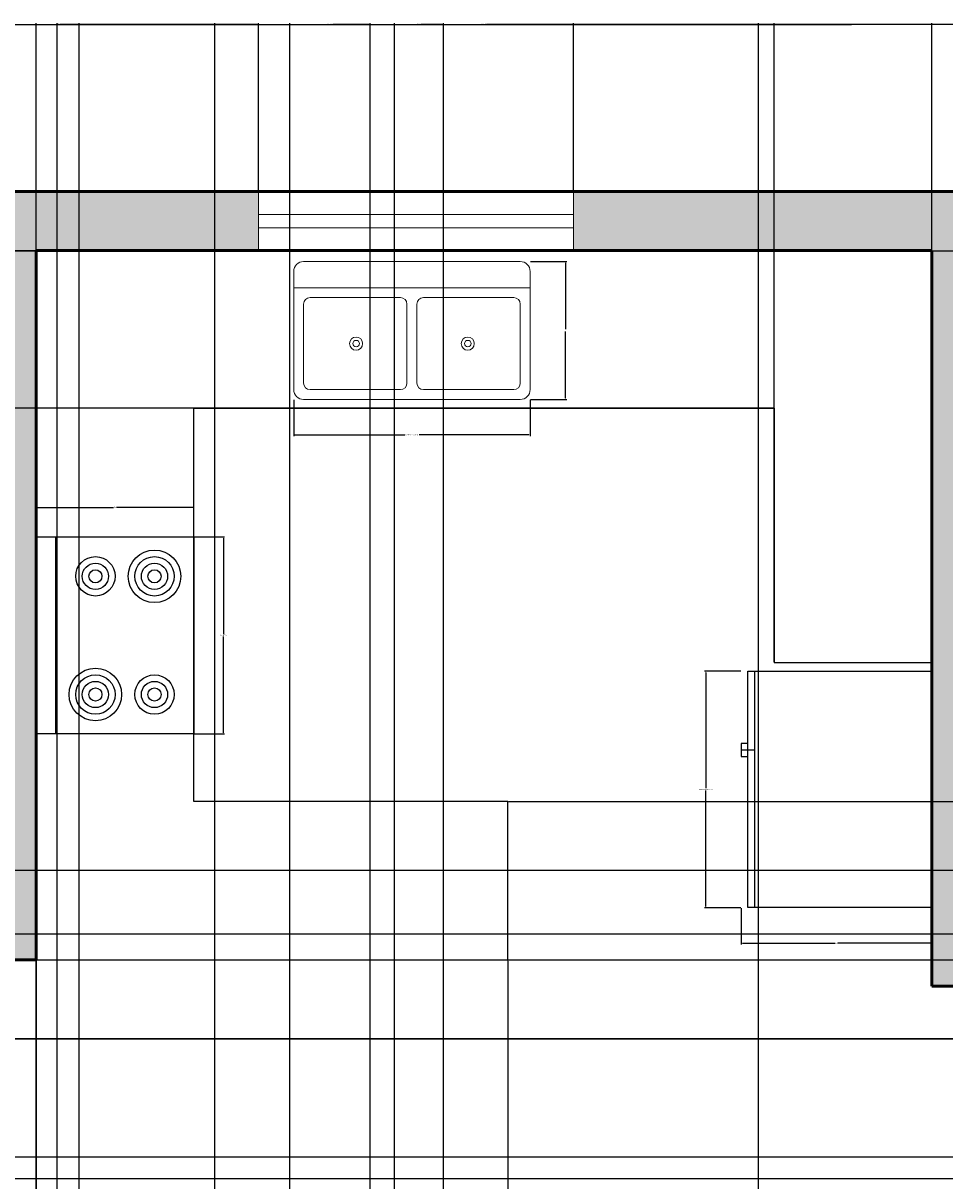
# Model space of a CAD drawing. Units: inches. Extents: x 3439 to 3988, y 1915 to 2284.
# Tile 6 of 7: x 3656 to 3796, y 2108 to 2284. Entities that reach past the tile are written whole.
import ezdxf

# ---------------------------------------------------------------- set-up
doc = ezdxf.new("R2010")
doc.units = ezdxf.units.IN
for name, color, linetype, lineweight in [('A-ANNO-DIMS', 2, 'Continuous', 18), ('A-EQPM', 8, 'Continuous', 25), ('A-FLOR-CASE', 8, 'Continuous', 25), ('A-FLOR-FIXT', 9, 'Continuous', 18), ('A-GLAZ', 4, 'Continuous', 18), ('A-WALL', 7, 'Continuous', 50)]:
    doc.layers.add(name, color=color, linetype=linetype, lineweight=lineweight)
doc.layers.add('A-WALL-PATT', color=18, linetype='Continuous', lineweight=13, true_color=0x000000)
doc.styles.get("Standard").update_dxf_attribs({"font": 'arial.ttf'})
doc.dimstyles.get("Standard").update_dxf_attribs({"dimtxt": 0.18, "dimasz": 0.18, "dimexe": 0.18, "dimexo": 0.0625, "dimgap": 0.09, "dimtad": 0, "dimtih": 1, "dimtoh": 1, "dimdec": 4, "dimzin": 0, "dimdsep": 46, "dimtxsty": 'Standard', "dimcen": 0.09, "dimadec": 0, "dimazin": 0, "dimtfac": 1, "dimtdec": 4, "dimtofl": 0, "dimtmove": 0, "dimatfit": 3, "dimfxl": 1, "dimtolj": 1, "dimtzin": 0, "dimarcsym": 0})

# ---------------------------------------------------------------- blocks, each defined once
blk = doc.blocks.new('Range-Oven - 30 in top')
blk.add_line((0, -3), (30, -3))
blk.add_lwpolyline([(0, -24), (0, 0), (30, 0), (30, -24)], close=True)
for centre, radius in [((6, -9), 4), ((6, -9), 3), ((6, -9), 2), ((24, -9), 3), ((24, -9), 2), ((6, -9), 1), ((24, -9), 1), ((24, -18), 4), ((6, -18), 3), ((24, -18), 3), ((6, -18), 2), ((6, -18), 1), ((24, -18), 2), ((24, -18), 1)]:
    blk.add_circle(centre, radius)
blk = doc.blocks.new('Sink-double - 36 in top')
for p, q in [((-18, -4), (18, -4)), ((-0.75, -18.5), (-0.75, -6.5)), ((0.75, -6.5), (0.75, -18.5))]:
    blk.add_line(p, q)
for points in [[(-16.5, 0), (16.5, 0)], [(-18, -19.5), (-18, -1.5)], [(18, -1.5), (18, -19.5)], [(-16.5, -18.5), (-16.5, -6.5)], [(-15.5, -5.5), (-1.75, -5.5)], [(1.75, -5.5), (15.5, -5.5)], [(16.5, -6.5), (16.5, -18.5)], [(16.5, -21), (-16.5, -21)], [(-1.75, -19.5), (-15.5, -19.5)], [(15.5, -19.5), (1.75, -19.5)]]:
    blk.add_lwpolyline(points)
for centre, radius in [((-8.5, -12.5), 1), ((-8.5, -12.5), 0.5), ((8.5, -12.5), 1), ((8.5, -12.5), 0.5)]:
    blk.add_circle(centre, radius)
for centre, radius, start, end in [((-16.5, -1.5), 1.5, 90, 180), ((16.5, -1.5), 1.5, 0, 90), ((-15.5, -6.5), 1, 90, 180), ((-1.75, -6.5), 1, 0, 90), ((1.75, -6.5), 1, 90, 180), ((15.5, -6.5), 1, 0, 90), ((-15.5, -18.5), 1, 180, 270), ((-1.75, -18.5), 1, 270, 0), ((1.75, -18.5), 1, 180, 270), ((15.5, -18.5), 1, 270, 0), ((-16.5, -19.5), 1.5, 180, 270), ((16.5, -19.5), 1.5, 270, 0)]:
    blk.add_arc(centre, radius, start, end)
blk = doc.blocks.new('Refrigerator-2 door - 36 in top')
for p, q in [((0, -26.999999), (36, -26.999999)), ((11, -27.999999), (11, -28.999999)), ((12, -26.999999), (12, -28.999999)), ((13, -28.999999), (13, -27.999999)), ((11, -28.999999), (13, -28.999999))]:
    blk.add_line(p, q)
blk.add_lwpolyline([(0, -27.999999), (0, 0), (36, 0), (36, -27.999999)], close=True)
blk = doc.blocks.new('WINDOW-GLASS-48IN')
for p, q in [((0, 2), (48, 2)), ((0, 0), (48, 0))]:
    blk.add_line(p, q)
blk = doc.blocks.new('*D37')
at = {"layer": 'A-ANNO-DIMS', "color": 0, "lineweight": -2, "transparency": 16777216}
for p, q in [((3681.64, 2205.78), (3686.26, 2205.78)), ((3686.08, 2205.6), (3686.08, 2190.96)), ((3686.08, 2175.96), (3686.08, 2190.59)), ((3681.64, 2175.78), (3686.26, 2175.78))]:
    blk.add_line(p, q, dxfattribs=at)
at = {"layer": 'A-ANNO-DIMS', "color": 0, "transparency": 16777216}
for points in [[(3686.05, 2205.6), (3686.11, 2205.6), (3686.08, 2205.78)], [(3686.05, 2175.96), (3686.11, 2175.96), (3686.08, 2175.78)]]:
    blk.add_solid(points, dxfattribs=at)
at = {"layer": 'Defpoints', "color": 0, "transparency": 16777216}
for p in [(3681.58, 2205.78), (3686.08, 2205.78), (3681.58, 2175.78)]:
    blk.add_point(p, dxfattribs=at)
at = {"layer": 'A-ANNO-DIMS', "color": 0, "transparency": 16777216, "insert": (3686.08, 2190.78), "char_height": 0.18, "attachment_point": 5}
blk.add_mtext('\\A1;RANGE 30', dxfattribs=at)
blk = doc.blocks.new('*D38')
at = {"layer": 'A-ANNO-DIMS', "color": 0, "lineweight": -2, "transparency": 16777216}
for p, q in [((3657.58, 2205.84), (3657.58, 2210.46)), ((3657.76, 2210.28), (3669.36, 2210.28)), ((3681.4, 2210.28), (3669.8, 2210.28)), ((3681.58, 2205.84), (3681.58, 2210.46))]:
    blk.add_line(p, q, dxfattribs=at)
at = {"layer": 'A-ANNO-DIMS', "color": 0, "transparency": 16777216}
for points in [[(3657.76, 2210.31), (3657.76, 2210.25), (3657.58, 2210.28)], [(3681.4, 2210.31), (3681.4, 2210.25), (3681.58, 2210.28)]]:
    blk.add_solid(points, dxfattribs=at)
at = {"layer": 'Defpoints', "color": 0, "transparency": 16777216}
for p in [(3657.58, 2210.28), (3657.58, 2205.78), (3681.58, 2205.78)]:
    blk.add_point(p, dxfattribs=at)
at = {"layer": 'A-ANNO-DIMS', "color": 0, "transparency": 16777216, "insert": (3669.58, 2210.28), "char_height": 0.18, "attachment_point": 5}
blk.add_mtext('\\A1;24', dxfattribs=at)
blk = doc.blocks.new('*D39')
at = {"layer": 'A-ANNO-DIMS', "color": 0, "lineweight": -2, "transparency": 16777216}
for p, q in [((3696.78, 2226.64), (3696.78, 2221.13)), ((3732.78, 2226.64), (3732.78, 2221.13)), ((3696.96, 2221.31), (3713.69, 2221.31)), ((3732.6, 2221.31), (3715.87, 2221.31))]:
    blk.add_line(p, q, dxfattribs=at)
at = {"layer": 'A-ANNO-DIMS', "color": 0, "transparency": 16777216}
for points in [[(3696.96, 2221.34), (3696.96, 2221.28), (3696.78, 2221.31)], [(3732.6, 2221.34), (3732.6, 2221.28), (3732.78, 2221.31)]]:
    blk.add_solid(points, dxfattribs=at)
at = {"layer": 'Defpoints', "color": 0, "transparency": 16777216}
for p in [(3696.78, 2226.71), (3732.78, 2226.71), (3732.78, 2221.31)]:
    blk.add_point(p, dxfattribs=at)
at = {"layer": 'A-ANNO-DIMS', "color": 0, "transparency": 16777216, "insert": (3714.78, 2221.31), "char_height": 0.18, "attachment_point": 5}
blk.add_mtext('\\A1;DOUBLE SINK 36', dxfattribs=at)
blk = doc.blocks.new('*D40')
at = {"layer": 'A-ANNO-DIMS', "color": 0, "lineweight": -2, "transparency": 16777216}
for p, q in [((3732.84, 2247.71), (3738.36, 2247.71)), ((3738.18, 2247.53), (3738.18, 2237.39)), ((3738.18, 2226.89), (3738.18, 2237.03)), ((3732.84, 2226.71), (3738.36, 2226.71))]:
    blk.add_line(p, q, dxfattribs=at)
at = {"layer": 'A-ANNO-DIMS', "color": 0, "transparency": 16777216}
for points in [[(3738.15, 2247.53), (3738.21, 2247.53), (3738.18, 2247.71)], [(3738.15, 2226.89), (3738.21, 2226.89), (3738.18, 2226.71)]]:
    blk.add_solid(points, dxfattribs=at)
at = {"layer": 'Defpoints', "color": 0, "transparency": 16777216}
for p in [(3732.78, 2247.71), (3738.18, 2247.71), (3732.78, 2226.71)]:
    blk.add_point(p, dxfattribs=at)
at = {"layer": 'A-ANNO-DIMS', "color": 0, "transparency": 16777216, "insert": (3738.18, 2237.21), "char_height": 0.18, "attachment_point": 5}
blk.add_mtext('\\A1;21', dxfattribs=at)
blk = doc.blocks.new('*D43')
at = {"layer": 'A-ANNO-DIMS', "color": 0, "lineweight": -2, "transparency": 16777216}
for p, q in [((3764.87, 2185.32), (3759.35, 2185.32)), ((3759.53, 2185.14), (3759.53, 2167.51)), ((3759.53, 2149.5), (3759.53, 2167.14)), ((3764.87, 2149.32), (3759.35, 2149.32))]:
    blk.add_line(p, q, dxfattribs=at)
at = {"layer": 'A-ANNO-DIMS', "color": 0, "transparency": 16777216}
for points in [[(3759.5, 2185.14), (3759.56, 2185.14), (3759.53, 2185.32)], [(3759.5, 2149.5), (3759.56, 2149.5), (3759.53, 2149.32)]]:
    blk.add_solid(points, dxfattribs=at)
at = {"layer": 'Defpoints', "color": 0, "transparency": 16777216}
for p in [(3764.93, 2185.32), (3759.53, 2149.32), (3764.93, 2149.32)]:
    blk.add_point(p, dxfattribs=at)
at = {"layer": 'A-ANNO-DIMS', "color": 0, "transparency": 16777216, "insert": (3759.53, 2167.32), "char_height": 0.18, "attachment_point": 5}
blk.add_mtext('\\A1;REFRIGERATOR 36', dxfattribs=at)
blk = doc.blocks.new('*D44')
at = {"layer": 'A-ANNO-DIMS', "color": 0, "lineweight": -2, "transparency": 16777216}
for p, q in [((3764.93, 2149.26), (3764.93, 2143.74)), ((3793.93, 2149.26), (3793.93, 2143.74)), ((3765.11, 2143.92), (3779.21, 2143.92)), ((3793.75, 2143.92), (3779.65, 2143.92))]:
    blk.add_line(p, q, dxfattribs=at)
at = {"layer": 'A-ANNO-DIMS', "color": 0, "transparency": 16777216}
for points in [[(3765.11, 2143.95), (3765.11, 2143.89), (3764.93, 2143.92)], [(3793.75, 2143.95), (3793.75, 2143.89), (3793.93, 2143.92)]]:
    blk.add_solid(points, dxfattribs=at)
at = {"layer": 'Defpoints', "color": 0, "transparency": 16777216}
for p in [(3764.93, 2149.32), (3793.93, 2149.32), (3793.93, 2143.92)]:
    blk.add_point(p, dxfattribs=at)
at = {"layer": 'A-ANNO-DIMS', "color": 0, "transparency": 16777216, "insert": (3779.43, 2143.92), "char_height": 0.18, "attachment_point": 5}
blk.add_mtext('\\A1;29', dxfattribs=at)
blk = doc.blocks.new('*D49')
at = {"layer": 'A-ANNO-DIMS', "color": 0, "lineweight": -2, "transparency": 16777216}
for p, q in [((3657.58, 2249.42), (3657.58, 2284)), ((3657.76, 2283.82), (3725.3, 2283.82)), ((3793.75, 2283.82), (3726.21, 2283.82)), ((3793.93, 2249.42), (3793.93, 2284))]:
    blk.add_line(p, q, dxfattribs=at)
at = {"layer": 'A-ANNO-DIMS', "color": 0, "transparency": 16777216}
for points in [[(3657.76, 2283.85), (3657.76, 2283.79), (3657.58, 2283.82)], [(3793.75, 2283.85), (3793.75, 2283.79), (3793.93, 2283.82)]]:
    blk.add_solid(points, dxfattribs=at)
at = {"layer": 'Defpoints', "color": 0, "transparency": 16777216}
for p in [(3793.93, 2283.82), (3657.58, 2249.36), (3793.93, 2249.36)]:
    blk.add_point(p, dxfattribs=at)
at = {"layer": 'A-ANNO-DIMS', "color": 0, "transparency": 16777216, "insert": (3725.76, 2283.82), "char_height": 0.18, "attachment_point": 5}
blk.add_mtext('\\A1;136.35', dxfattribs=at)
blk = doc.blocks.new('*D64')
at = {"layer": 'A-ANNO-DIMS', "color": 0, "lineweight": -2, "transparency": 16777216}
for p, q in [((3593.64, 2249.36), (3987.81, 2249.36)), ((3987.63, 2249.18), (3987.63, 2197.54)), ((3987.63, 2145.54), (3987.63, 2197.18)), ((3593.64, 2145.36), (3987.81, 2145.36))]:
    blk.add_line(p, q, dxfattribs=at)
at = {"layer": 'A-ANNO-DIMS', "color": 0, "transparency": 16777216}
for points in [[(3987.6, 2249.18), (3987.66, 2249.18), (3987.63, 2249.36)], [(3987.6, 2145.54), (3987.66, 2145.54), (3987.63, 2145.36)]]:
    blk.add_solid(points, dxfattribs=at)
at = {"layer": 'Defpoints', "color": 0, "transparency": 16777216}
for p in [(3593.58, 2249.36), (3987.63, 2249.36), (3593.58, 2145.36)]:
    blk.add_point(p, dxfattribs=at)
at = {"layer": 'A-ANNO-DIMS', "color": 0, "transparency": 16777216, "insert": (3987.63, 2197.36), "char_height": 0.18, "attachment_point": 5}
blk.add_mtext('\\A1;104', dxfattribs=at)
blk = doc.blocks.new('*D68')
at = {"layer": 'A-ANNO-DIMS', "color": 0, "lineweight": -2, "transparency": 16777216}
for p, q in [((3631.59, 2258.42), (3631.59, 2284)), ((3631.77, 2283.82), (3661.12, 2283.82)), ((3691.23, 2283.82), (3661.88, 2283.82)), ((3691.41, 2258.42), (3691.41, 2284))]:
    blk.add_line(p, q, dxfattribs=at)
at = {"layer": 'A-ANNO-DIMS', "color": 0, "transparency": 16777216}
for points in [[(3631.77, 2283.85), (3631.77, 2283.79), (3631.59, 2283.82)], [(3691.23, 2283.85), (3691.23, 2283.79), (3691.41, 2283.82)]]:
    blk.add_solid(points, dxfattribs=at)
at = {"layer": 'Defpoints', "color": 0, "transparency": 16777216}
for p in [(3691.41, 2283.82), (3631.59, 2258.36), (3691.41, 2258.36)]:
    blk.add_point(p, dxfattribs=at)
at = {"layer": 'A-ANNO-DIMS', "color": 0, "transparency": 16777216, "insert": (3661.5, 2283.82), "char_height": 0.18, "attachment_point": 5}
blk.add_mtext('\\A1;59.81', dxfattribs=at)
blk = doc.blocks.new('*D69')
at = {"layer": 'A-ANNO-DIMS', "color": 0, "lineweight": -2, "transparency": 16777216}
for p, q in [((3739.41, 2258.42), (3739.41, 2284)), ((3739.59, 2283.82), (3771.27, 2283.82)), ((3803.75, 2283.82), (3772.06, 2283.82)), ((3803.93, 2258.42), (3803.93, 2284))]:
    blk.add_line(p, q, dxfattribs=at)
at = {"layer": 'A-ANNO-DIMS', "color": 0, "transparency": 16777216}
for points in [[(3739.59, 2283.85), (3739.59, 2283.79), (3739.41, 2283.82)], [(3803.75, 2283.85), (3803.75, 2283.79), (3803.93, 2283.82)]]:
    blk.add_solid(points, dxfattribs=at)
at = {"layer": 'Defpoints', "color": 0, "transparency": 16777216}
for p in [(3803.93, 2283.82), (3739.41, 2258.36), (3803.93, 2258.36)]:
    blk.add_point(p, dxfattribs=at)
at = {"layer": 'A-ANNO-DIMS', "color": 0, "transparency": 16777216, "insert": (3771.67, 2283.82), "char_height": 0.18, "attachment_point": 5}
blk.add_mtext('\\A1;64.53', dxfattribs=at)
blk = doc.blocks.new('*D73')
at = {"layer": 'A-ANNO-DIMS', "color": 0, "lineweight": -2, "transparency": 16777216}
for p, q in [((3657.58, 1949.42), (3657.58, 2284)), ((3657.76, 2283.82), (3660.52, 2283.82)), ((3663.93, 2283.82), (3661.17, 2283.82)), ((3664.11, 1949.42), (3664.11, 2284))]:
    blk.add_line(p, q, dxfattribs=at)
at = {"layer": 'A-ANNO-DIMS', "color": 0, "transparency": 16777216}
for points in [[(3657.76, 2283.85), (3657.76, 2283.79), (3657.58, 2283.82)], [(3663.93, 2283.85), (3663.93, 2283.79), (3664.11, 2283.82)]]:
    blk.add_solid(points, dxfattribs=at)
at = {"layer": 'Defpoints', "color": 0, "transparency": 16777216}
for p in [(3664.11, 2283.82), (3657.58, 1949.36), (3664.11, 1949.36)]:
    blk.add_point(p, dxfattribs=at)
at = {"layer": 'A-ANNO-DIMS', "color": 0, "transparency": 16777216, "insert": (3660.85, 2283.82), "char_height": 0.18, "attachment_point": 5}
blk.add_mtext('\\A1;6.53', dxfattribs=at)
blk = doc.blocks.new('*D74')
at = {"layer": 'A-ANNO-DIMS', "color": 0, "lineweight": -2, "transparency": 16777216}
for p, q in [((3712.11, 1949.42), (3712.11, 2284)), ((3712.29, 2283.82), (3715.52, 2283.82)), ((3719.4, 2283.82), (3716.17, 2283.82)), ((3719.58, 1949.42), (3719.58, 2284))]:
    blk.add_line(p, q, dxfattribs=at)
at = {"layer": 'A-ANNO-DIMS', "color": 0, "transparency": 16777216}
for points in [[(3712.29, 2283.85), (3712.29, 2283.79), (3712.11, 2283.82)], [(3719.4, 2283.85), (3719.4, 2283.79), (3719.58, 2283.82)]]:
    blk.add_solid(points, dxfattribs=at)
at = {"layer": 'Defpoints', "color": 0, "transparency": 16777216}
for p in [(3719.58, 2283.82), (3712.11, 1949.36), (3719.58, 1949.36)]:
    blk.add_point(p, dxfattribs=at)
at = {"layer": 'A-ANNO-DIMS', "color": 0, "transparency": 16777216, "insert": (3715.85, 2283.82), "char_height": 0.18, "attachment_point": 5}
blk.add_mtext('\\A1;7.47', dxfattribs=at)
blk = doc.blocks.new('*D75')
at = {"layer": 'A-ANNO-DIMS', "color": 0, "lineweight": -2, "transparency": 16777216}
for p, q in [((3719.58, 1949.42), (3719.58, 2284)), ((3719.76, 2283.82), (3743.36, 2283.82)), ((3767.4, 2283.82), (3743.8, 2283.82)), ((3767.58, 1949.42), (3767.58, 2284))]:
    blk.add_line(p, q, dxfattribs=at)
at = {"layer": 'A-ANNO-DIMS', "color": 0, "transparency": 16777216}
for points in [[(3719.76, 2283.85), (3719.76, 2283.79), (3719.58, 2283.82)], [(3767.4, 2283.85), (3767.4, 2283.79), (3767.58, 2283.82)]]:
    blk.add_solid(points, dxfattribs=at)
at = {"layer": 'Defpoints', "color": 0, "transparency": 16777216}
for p in [(3767.58, 2283.82), (3719.58, 1949.36), (3767.58, 1949.36)]:
    blk.add_point(p, dxfattribs=at)
at = {"layer": 'A-ANNO-DIMS', "color": 0, "transparency": 16777216, "insert": (3743.58, 2283.82), "char_height": 0.18, "attachment_point": 5}
blk.add_mtext('\\A1;48', dxfattribs=at)
blk = doc.blocks.new('*D77')
at = {"layer": 'A-ANNO-DIMS', "color": 0, "lineweight": -2, "transparency": 16777216}
for p, q in [((3473.64, 2129.36), (3987.81, 2129.36)), ((3987.63, 2129.18), (3987.63, 2118.9)), ((3987.63, 2108.25), (3987.63, 2118.53)), ((3473.64, 2108.07), (3987.81, 2108.07))]:
    blk.add_line(p, q, dxfattribs=at)
at = {"layer": 'A-ANNO-DIMS', "color": 0, "transparency": 16777216}
for points in [[(3987.6, 2129.18), (3987.66, 2129.18), (3987.63, 2129.36)], [(3987.6, 2108.25), (3987.66, 2108.25), (3987.63, 2108.07)]]:
    blk.add_solid(points, dxfattribs=at)
at = {"layer": 'Defpoints', "color": 0, "transparency": 16777216}
for p in [(3473.58, 2129.36), (3987.63, 2129.36), (3473.58, 2108.07)]:
    blk.add_point(p, dxfattribs=at)
at = {"layer": 'A-ANNO-DIMS', "color": 0, "transparency": 16777216, "insert": (3987.63, 2118.71), "char_height": 0.18, "attachment_point": 5}
blk.add_mtext('\\A1;21.295', dxfattribs=at)
blk = doc.blocks.new('*D82')
at = {"layer": 'A-ANNO-DIMS', "color": 0, "lineweight": -2, "transparency": 16777216}
for p, q in [((3537.64, 2129.36), (3987.81, 2129.36)), ((3987.63, 2129.18), (3987.63, 2120.54)), ((3987.63, 2111.54), (3987.63, 2120.18)), ((3537.64, 2111.36), (3987.81, 2111.36))]:
    blk.add_line(p, q, dxfattribs=at)
at = {"layer": 'A-ANNO-DIMS', "color": 0, "transparency": 16777216}
for points in [[(3987.6, 2129.18), (3987.66, 2129.18), (3987.63, 2129.36)], [(3987.6, 2111.54), (3987.66, 2111.54), (3987.63, 2111.36)]]:
    blk.add_solid(points, dxfattribs=at)
at = {"layer": 'Defpoints', "color": 0, "transparency": 16777216}
for p in [(3537.58, 2129.36), (3987.63, 2129.36), (3537.58, 2111.36)]:
    blk.add_point(p, dxfattribs=at)
at = {"layer": 'A-ANNO-DIMS', "color": 0, "transparency": 16777216, "insert": (3987.63, 2120.36), "char_height": 0.18, "attachment_point": 5}
blk.add_mtext('\\A1;18', dxfattribs=at)
blk = doc.blocks.new('*D83')
at = {"layer": 'A-ANNO-DIMS', "color": 0, "lineweight": -2, "transparency": 16777216}
for p, q in [((3537.64, 2111.36), (3987.81, 2111.36)), ((3987.63, 2111.18), (3987.63, 2099.54)), ((3987.63, 2087.54), (3987.63, 2099.18)), ((3537.64, 2087.36), (3987.81, 2087.36))]:
    blk.add_line(p, q, dxfattribs=at)
at = {"layer": 'A-ANNO-DIMS', "color": 0, "transparency": 16777216}
for points in [[(3987.6, 2111.18), (3987.66, 2111.18), (3987.63, 2111.36)], [(3987.6, 2087.54), (3987.66, 2087.54), (3987.63, 2087.36)]]:
    blk.add_solid(points, dxfattribs=at)
at = {"layer": 'Defpoints', "color": 0, "transparency": 16777216}
for p in [(3537.58, 2111.36), (3987.63, 2111.36), (3537.58, 2087.36)]:
    blk.add_point(p, dxfattribs=at)
at = {"layer": 'A-ANNO-DIMS', "color": 0, "transparency": 16777216, "insert": (3987.63, 2099.36), "char_height": 0.18, "attachment_point": 5}
blk.add_mtext('\\A1;24', dxfattribs=at)
blk = doc.blocks.new('*D94')
at = {"layer": 'A-ANNO-DIMS', "color": 0, "lineweight": -2, "transparency": 16777216}
for p, q in [((3657.58, 2141.3), (3657.58, 1915.13)), ((3729.41, 2141.3), (3729.41, 1915.13)), ((3657.76, 1915.31), (3693.1, 1915.31)), ((3729.23, 1915.31), (3693.89, 1915.31))]:
    blk.add_line(p, q, dxfattribs=at)
at = {"layer": 'A-ANNO-DIMS', "color": 0, "transparency": 16777216}
for points in [[(3657.76, 1915.34), (3657.76, 1915.28), (3657.58, 1915.31)], [(3729.23, 1915.34), (3729.23, 1915.28), (3729.41, 1915.31)]]:
    blk.add_solid(points, dxfattribs=at)
at = {"layer": 'Defpoints', "color": 0, "transparency": 16777216}
for p in [(3657.58, 2141.36), (3729.41, 2141.36), (3729.41, 1915.31)]:
    blk.add_point(p, dxfattribs=at)
at = {"layer": 'A-ANNO-DIMS', "color": 0, "transparency": 16777216, "insert": (3693.49, 1915.31), "char_height": 0.18, "attachment_point": 5}
blk.add_mtext('\\A1;71.83', dxfattribs=at)
blk = doc.blocks.new('*D95')
at = {"layer": 'A-ANNO-DIMS', "color": 0, "lineweight": -2, "transparency": 16777216}
for p, q in [((3729.47, 2165.5), (3987.81, 2165.5)), ((3987.63, 2165.32), (3987.63, 2153.61)), ((3987.63, 2141.54), (3987.63, 2153.25)), ((3729.47, 2141.36), (3987.81, 2141.36))]:
    blk.add_line(p, q, dxfattribs=at)
at = {"layer": 'A-ANNO-DIMS', "color": 0, "transparency": 16777216}
for points in [[(3987.6, 2165.32), (3987.66, 2165.32), (3987.63, 2165.5)], [(3987.6, 2141.54), (3987.66, 2141.54), (3987.63, 2141.36)]]:
    blk.add_solid(points, dxfattribs=at)
at = {"layer": 'Defpoints', "color": 0, "transparency": 16777216}
for p in [(3729.41, 2165.5), (3987.63, 2165.5), (3729.41, 2141.36)]:
    blk.add_point(p, dxfattribs=at)
at = {"layer": 'A-ANNO-DIMS', "color": 0, "transparency": 16777216, "insert": (3987.63, 2153.43), "char_height": 0.18, "attachment_point": 5}
blk.add_mtext('\\A1;24.14', dxfattribs=at)
blk = doc.blocks.new('*D96')
at = {"layer": 'A-ANNO-DIMS', "color": 0, "lineweight": -2, "transparency": 16777216}
for p, q in [((3793.87, 2249.36), (3439.35, 2249.36)), ((3439.53, 2249.18), (3439.53, 2237.54)), ((3439.53, 2225.54), (3439.53, 2237.18)), ((3769.87, 2225.36), (3439.35, 2225.36))]:
    blk.add_line(p, q, dxfattribs=at)
at = {"layer": 'A-ANNO-DIMS', "color": 0, "transparency": 16777216}
for points in [[(3439.5, 2249.18), (3439.56, 2249.18), (3439.53, 2249.36)], [(3439.5, 2225.54), (3439.56, 2225.54), (3439.53, 2225.36)]]:
    blk.add_solid(points, dxfattribs=at)
at = {"layer": 'Defpoints', "color": 0, "transparency": 16777216}
for p in [(3439.53, 2249.36), (3793.93, 2249.36), (3769.93, 2225.36)]:
    blk.add_point(p, dxfattribs=at)
at = {"layer": 'A-ANNO-DIMS', "color": 0, "transparency": 16777216, "insert": (3439.53, 2237.36), "char_height": 0.18, "attachment_point": 5}
blk.add_mtext('\\A1;24', dxfattribs=at)
blk = doc.blocks.new('*D97')
at = {"layer": 'A-ANNO-DIMS', "color": 0, "lineweight": -2, "transparency": 16777216}
for p, q in [((3769.93, 2186.73), (3769.93, 2284)), ((3770.11, 2283.82), (3781.71, 2283.82)), ((3793.75, 2283.82), (3782.15, 2283.82)), ((3793.93, 2186.73), (3793.93, 2284))]:
    blk.add_line(p, q, dxfattribs=at)
at = {"layer": 'A-ANNO-DIMS', "color": 0, "transparency": 16777216}
for points in [[(3770.11, 2283.85), (3770.11, 2283.79), (3769.93, 2283.82)], [(3793.75, 2283.85), (3793.75, 2283.79), (3793.93, 2283.82)]]:
    blk.add_solid(points, dxfattribs=at)
at = {"layer": 'Defpoints', "color": 0, "transparency": 16777216}
for p in [(3793.93, 2283.82), (3769.93, 2186.66), (3793.93, 2186.66)]:
    blk.add_point(p, dxfattribs=at)
at = {"layer": 'A-ANNO-DIMS', "color": 0, "transparency": 16777216, "insert": (3781.93, 2283.82), "char_height": 0.18, "attachment_point": 5}
blk.add_mtext('\\A1;24', dxfattribs=at)
blk = doc.blocks.new('*D98')
at = {"layer": 'A-ANNO-DIMS', "color": 0, "lineweight": -2, "transparency": 16777216}
for p, q in [((3889.52, 2154.99), (3439.35, 2154.99)), ((3439.53, 2154.81), (3439.53, 2142.36)), ((3439.53, 2129.54), (3439.53, 2141.99)), ((3889.52, 2129.36), (3439.35, 2129.36))]:
    blk.add_line(p, q, dxfattribs=at)
at = {"layer": 'A-ANNO-DIMS', "color": 0, "transparency": 16777216}
for points in [[(3439.5, 2154.81), (3439.56, 2154.81), (3439.53, 2154.99)], [(3439.5, 2129.54), (3439.56, 2129.54), (3439.53, 2129.36)]]:
    blk.add_solid(points, dxfattribs=at)
at = {"layer": 'Defpoints', "color": 0, "transparency": 16777216}
for p in [(3889.58, 2154.99), (3439.53, 2129.36), (3889.58, 2129.36)]:
    blk.add_point(p, dxfattribs=at)
at = {"layer": 'A-ANNO-DIMS', "color": 0, "transparency": 16777216, "insert": (3439.53, 2142.18), "char_height": 0.18, "attachment_point": 5}
blk.add_mtext('\\A1;25.63', dxfattribs=at)
blk = doc.blocks.new('*D99')
at = {"layer": 'A-ANNO-DIMS', "color": 0, "lineweight": -2, "transparency": 16777216}
for p, q in [((3660.76, 2019.79), (3660.76, 2284)), ((3660.94, 2283.82), (3672.54, 2283.82)), ((3684.58, 2283.82), (3672.98, 2283.82)), ((3684.76, 2019.79), (3684.76, 2284))]:
    blk.add_line(p, q, dxfattribs=at)
at = {"layer": 'A-ANNO-DIMS', "color": 0, "transparency": 16777216}
for points in [[(3660.94, 2283.85), (3660.94, 2283.79), (3660.76, 2283.82)], [(3684.58, 2283.85), (3684.58, 2283.79), (3684.76, 2283.82)]]:
    blk.add_solid(points, dxfattribs=at)
at = {"layer": 'Defpoints', "color": 0, "transparency": 16777216}
for p in [(3684.76, 2283.82), (3660.76, 2019.72), (3684.76, 2019.72)]:
    blk.add_point(p, dxfattribs=at)
at = {"layer": 'A-ANNO-DIMS', "color": 0, "transparency": 16777216, "insert": (3672.76, 2283.82), "char_height": 0.18, "attachment_point": 5}
blk.add_mtext('\\A1;24', dxfattribs=at)
blk = doc.blocks.new('*D101')
at = {"layer": 'A-ANNO-DIMS', "color": 0, "lineweight": -2, "transparency": 16777216}
for p, q in [((3696.21, 2004.22), (3696.21, 2284)), ((3696.39, 2283.82), (3701.86, 2283.82)), ((3708.24, 2283.82), (3702.77, 2283.82)), ((3708.42, 2004.22), (3708.42, 2284))]:
    blk.add_line(p, q, dxfattribs=at)
at = {"layer": 'A-ANNO-DIMS', "color": 0, "transparency": 16777216}
for points in [[(3696.39, 2283.85), (3696.39, 2283.79), (3696.21, 2283.82)], [(3708.24, 2283.85), (3708.24, 2283.79), (3708.42, 2283.82)]]:
    blk.add_solid(points, dxfattribs=at)
at = {"layer": 'Defpoints', "color": 0, "transparency": 16777216}
for p in [(3708.42, 2283.82), (3696.21, 2004.16), (3708.42, 2004.16)]:
    blk.add_point(p, dxfattribs=at)
at = {"layer": 'A-ANNO-DIMS', "color": 0, "transparency": 16777216, "insert": (3702.31, 2283.82), "char_height": 0.18, "attachment_point": 5}
blk.add_mtext('\\A1;12.214', dxfattribs=at)

msp = doc.modelspace()

# ---------------------------------------------------------------- hatches: boundary and pattern name
at = {"layer": 'A-WALL-PATT'}
h = msp.add_hatch(color=256, dxfattribs=at)
h.dxf.hatch_style = 1
h.paths.add_polyline_path([(3691.4053, 2258.3617), (3631.5949, 2258.3617), (3631.5949, 2249.3617), (3653.5815, 2249.3617), (3653.5815, 2145.3617), (3623.5815, 2145.3617), (3623.5815, 2141.3617), (3657.5815, 2141.3617), (3657.5815, 2249.3617), (3691.4053, 2249.3617)])
h = msp.add_hatch(color=256, dxfattribs=at)
h.dxf.hatch_style = 1
h.paths.add_polyline_path([(3803.9319, 2258.3617), (3739.4053, 2258.3617), (3739.4053, 2249.3617), (3793.9319, 2249.3617), (3793.9319, 2137.3617), (3845.9319, 2137.3617), (3845.9319, 2125.3617), (3855.9319, 2125.3617), (3855.9319, 2129.3617), (3849.9319, 2129.3617), (3849.9319, 2249.3617), (3881.3564, 2249.3617), (3881.3564, 2258.3617), (3827.9319, 2258.3617), (3827.9319, 2249.3617), (3845.9319, 2249.3617), (3845.9319, 2141.3617), (3797.9319, 2141.3617), (3797.9319, 2249.3617), (3803.9319, 2249.3617)])

# ---------------------------------------------------------------- linework, layer by layer
at = {"layer": 'A-FLOR-CASE'}
for p, q in [((3681.5815, 2225.3617), (3769.9319, 2225.3617)), ((3681.5815, 2165.5018), (3681.5815, 2225.3617)), ((3769.9319, 2225.3617), (3769.9319, 2186.6628)), ((3769.9319, 2186.6628), (3793.9319, 2186.6628)), ((3729.4075, 2165.5018), (3681.5815, 2165.5018)), ((3729.4075, 2141.3617), (3729.4075, 2165.5018)), ((3657.5815, 2141.3617), (3729.4075, 2141.3617))]:
    msp.add_line(p, q, dxfattribs=at)
at = {"layer": 'A-GLAZ'}
for points in [[(3691.4053, 2249.3617), (3691.4053, 2258.3617)], [(3739.4053, 2258.3617), (3739.4053, 2249.3617)]]:
    msp.add_lwpolyline(points, dxfattribs=at)
at = {"layer": 'A-WALL'}
for p, q in [((3657.5815, 2249.3617), (3793.9319, 2249.3617)), ((3657.5815, 2141.3617), (3657.5815, 2249.3617)), ((3793.9319, 2249.3617), (3793.9319, 2137.3617)), ((3623.5815, 2141.3617), (3657.5815, 2141.3617)), ((3793.9319, 2137.3617), (3845.9319, 2137.3617))]:
    msp.add_line(p, q, dxfattribs=at)
msp.add_lwpolyline([(3719.5815, 1940.3617), (3464.5815, 1940.3617), (3464.5815, 2258.3617), (3803.9319, 2258.3617)], dxfattribs=at)

# ---------------------------------------------------------------- block references
at = {"layer": 'A-EQPM'}
for name, p, rotation in [('Range-Oven - 30 in top', (3657.5815, 2175.7768), 90), ('Refrigerator-2 door - 36 in top', (3793.9319, 2185.3244), 270)]:
    msp.add_blockref(name, p, dxfattribs=dict(at, rotation=rotation))
at = {"layer": 'A-FLOR-FIXT'}
msp.add_blockref('Sink-double - 36 in top', (3714.7799, 2247.7064), dxfattribs=at)
at = {"layer": 'A-GLAZ'}
msp.add_blockref('WINDOW-GLASS-48IN', (3691.4053, 2252.8617), dxfattribs=at)

# ---------------------------------------------------------------- dimensions: what is measured, and where the dimension line sits
at = {"layer": 'A-ANNO-DIMS'}
for base, p1, p2, override, picture, middle in [((3691.4053, 2283.8228), (3631.5949, 2258.3617), (3691.4053, 2258.3617), {"dimdec": 2, "dimlfac": 1, "dimrnd": 0, "dimzin": 0, "dimdsep": 46, "dimlunit": 2}, '*D68', (3661.5001, 2283.8228)), ((3793.9319, 2283.8228), (3657.5815, 2249.3617), (3793.9319, 2249.3617), {"dimdec": 2, "dimlfac": 1, "dimrnd": 0, "dimzin": 0, "dimdsep": 46, "dimlunit": 2}, '*D49', (3725.7567, 2283.8228)), ((3664.1118, 2283.8228), (3657.5815, 1949.3617), (3664.1118, 1949.3617), {"dimdec": 2, "dimlfac": 1, "dimrnd": 0, "dimzin": 0, "dimdsep": 46, "dimlunit": 2}, '*D73', (3660.8466, 2283.8228)), ((3684.7646, 2283.8228), (3660.7646, 2019.7238), (3684.7646, 2019.7238), {"dimdec": 0, "dimlfac": 1, "dimrnd": 0, "dimzin": 0, "dimdsep": 46, "dimlunit": 2}, '*D99', (3672.7646, 2283.8228)), ((3708.4216, 2283.8228), (3696.2076, 2004.1572), (3708.4216, 2004.1572), {"dimdec": 3, "dimlfac": 1, "dimrnd": 0, "dimzin": 0, "dimdsep": 46, "dimlunit": 2}, '*D101', (3702.3146, 2283.8228)), ((3719.5815, 2283.8228), (3712.1118, 1949.3617), (3719.5815, 1949.3617), {"dimdec": 2, "dimlfac": 1, "dimrnd": 0, "dimzin": 0, "dimdsep": 46, "dimlunit": 2}, '*D74', (3715.8466, 2283.8228)), ((3767.5815, 2283.8228), (3719.5815, 1949.3617), (3767.5815, 1949.3617), {"dimdec": 0, "dimlfac": 1, "dimrnd": 0, "dimzin": 0, "dimdsep": 46, "dimlunit": 2}, '*D75', (3743.5815, 2283.8228)), ((3803.9319, 2283.8228), (3739.4053, 2258.3617), (3803.9319, 2258.3617), {"dimdec": 2, "dimlfac": 1, "dimrnd": 0, "dimzin": 0, "dimdsep": 46, "dimlunit": 2}, '*D69', (3771.6686, 2283.8228)), ((3793.9319, 2283.8228), (3769.9319, 2186.6628), (3793.9319, 2186.6628), {"dimdec": 0, "dimlfac": 1, "dimrnd": 0, "dimzin": 0, "dimdsep": 46, "dimlunit": 2}, '*D97', (3781.9319, 2283.8228)), ((3793.9319, 2143.9244), (3764.9319, 2149.3244), (3793.9319, 2149.3244), {"dimdec": 0, "dimlfac": 1, "dimrnd": 0, "dimzin": 0, "dimdsep": 46, "dimlunit": 2}, '*D44', (3779.4319, 2143.9244)), ((3729.4075, 1915.3117), (3657.5815, 2141.3617), (3729.4075, 2141.3617), {"dimdec": 2, "dimlfac": 1, "dimrnd": 0, "dimzin": 0, "dimdsep": 46, "dimlunit": 2}, '*D94', (3693.4945, 1915.3117))]:
    dim = msp.add_linear_dim(base=base, p1=p1, p2=p2, dimstyle='Standard', override=override, dxfattribs=at)
    dim.commit()
    dim.dimension.update_dxf_attribs({"geometry": picture, "text_midpoint": middle})
for base, p1, p2, angle, override, picture, middle in [((3439.5315, 2249.3617), (3769.9319, 2225.3617), (3793.9319, 2249.3617), 90, {"dimdec": 0, "dimlfac": 1, "dimrnd": 0, "dimzin": 0, "dimdsep": 46, "dimlunit": 2}, '*D96', (3439.5315, 2237.3617)), ((3987.6315, 2249.3617), (3593.5815, 2145.3617), (3593.5815, 2249.3617), 90, {"dimdec": 0, "dimlfac": 1, "dimrnd": 0, "dimzin": 0, "dimdsep": 46, "dimlunit": 2}, '*D64', (3987.6315, 2197.3617)), ((3738.1799, 2247.7064), (3732.7799, 2226.7064), (3732.7799, 2247.7064), 90, {"dimdec": 0, "dimlfac": 1, "dimrnd": 0, "dimzin": 0, "dimdsep": 46, "dimlunit": 2}, '*D40', (3738.1799, 2237.2064)), ((3657.5815, 2210.2768), (3681.5815, 2205.7768), (3657.5815, 2205.7768), 180, {"dimdec": 0, "dimlfac": 1, "dimrnd": 0, "dimzin": 0, "dimdsep": 46, "dimlunit": 2}, '*D38', (3669.5815, 2210.2768)), ((3987.6315, 2165.5018), (3729.4075, 2141.3617), (3729.4075, 2165.5018), 90, {"dimdec": 2, "dimlfac": 1, "dimrnd": 0, "dimzin": 0, "dimdsep": 46, "dimlunit": 2}, '*D95', (3987.6315, 2153.4318)), ((3439.5315, 2129.3617), (3889.5815, 2154.9906), (3889.5815, 2129.3617), 90, {"dimdec": 2, "dimlfac": 1, "dimrnd": 0, "dimzin": 0, "dimdsep": 46, "dimlunit": 2}, '*D98', (3439.5315, 2142.1761)), ((3987.6315, 2129.3617), (3473.5815, 2108.0664), (3473.5815, 2129.3617), 90, {"dimdec": 3, "dimlfac": 1, "dimrnd": 0, "dimzin": 0, "dimdsep": 46, "dimlunit": 2}, '*D77', (3987.6315, 2118.7141)), ((3987.6315, 2129.3617), (3537.5815, 2111.3617), (3537.5815, 2129.3617), 90, {"dimdec": 0, "dimlfac": 1, "dimrnd": 0, "dimzin": 0, "dimdsep": 46, "dimlunit": 2}, '*D82', (3987.6315, 2120.3617)), ((3987.6315, 2111.3617), (3537.5815, 2087.3617), (3537.5815, 2111.3617), 90, {"dimdec": 0, "dimlfac": 1, "dimrnd": 0, "dimzin": 0, "dimdsep": 46, "dimlunit": 2}, '*D83', (3987.6315, 2099.3617))]:
    dim = msp.add_linear_dim(base=base, p1=p1, p2=p2, angle=angle, dimstyle='Standard', override=override, dxfattribs=at)
    dim.commit()
    dim.dimension.update_dxf_attribs({"geometry": picture, "text_midpoint": middle})
dim = msp.add_linear_dim(base=(3732.7799, 2221.3064), p1=(3696.7799, 2226.7064), p2=(3732.7799, 2226.7064), text='DOUBLE SINK <>', dimstyle='Standard', override={"dimdec": 0, "dimlfac": 1, "dimrnd": 0, "dimzin": 0, "dimdsep": 46, "dimlunit": 2}, dxfattribs=at)
dim.commit()
dim.dimension.update_dxf_attribs({"geometry": '*D39', "text_midpoint": (3714.7799, 2221.3064)})
for base, p1, p2, angle, text, picture, middle in [((3686.0815, 2205.7768), (3681.5815, 2175.7768), (3681.5815, 2205.7768), 90, 'RANGE <>', '*D37', (3686.0815, 2190.7768)), ((3759.5319, 2149.3244), (3764.9319, 2185.3244), (3764.9319, 2149.3244), 270, 'REFRIGERATOR <>', '*D43', (3759.5319, 2167.3244))]:
    dim = msp.add_linear_dim(base=base, p1=p1, p2=p2, angle=angle, text=text, dimstyle='Standard', override={"dimdec": 0, "dimlfac": 1, "dimrnd": 0, "dimzin": 0, "dimdsep": 46, "dimlunit": 2}, dxfattribs=at)
    dim.commit()
    dim.dimension.update_dxf_attribs({"geometry": picture, "text_midpoint": middle})

doc.saveas('drawing.dxf')
